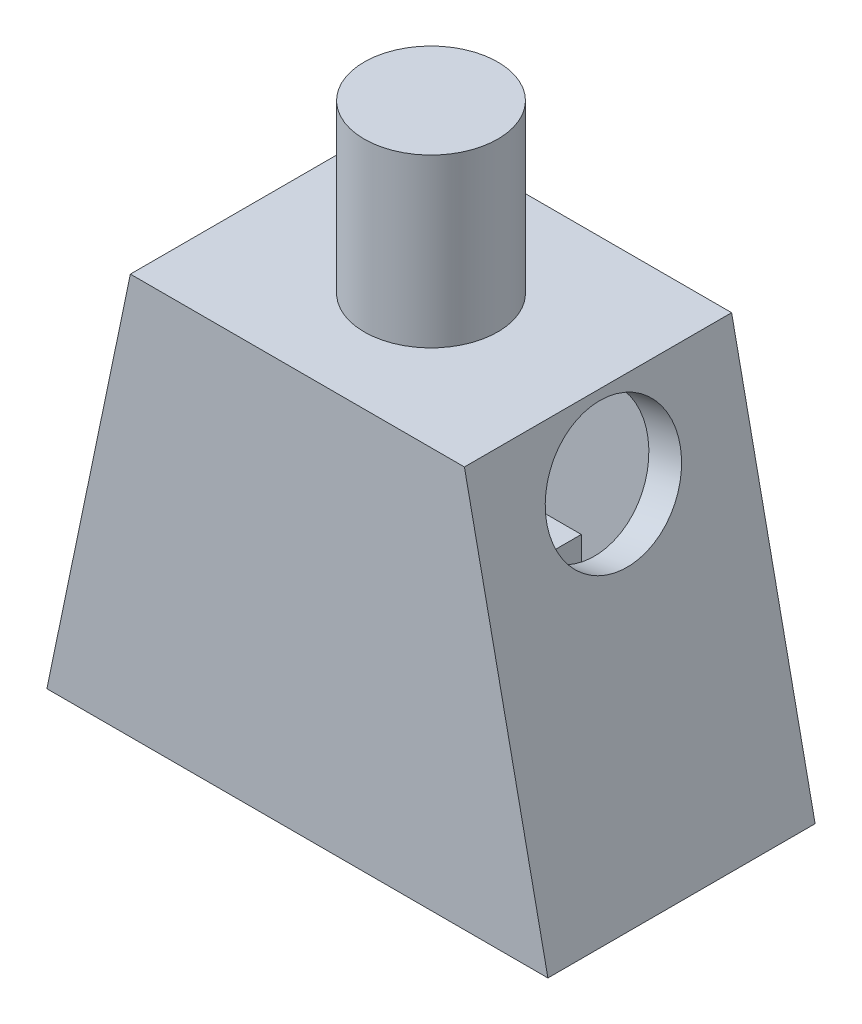
ISO-10303-21;
HEADER;
FILE_DESCRIPTION(('STEP AP214'),'2;1');
FILE_NAME('part.step','',(''),(''),'','','');
FILE_SCHEMA(('AUTOMOTIVE_DESIGN { 1 0 10303 214 1 1 1 1 }'));
ENDSEC;
DATA;
#1=APPLICATION_CONTEXT('core data for automotive mechanical design processes');
#2=APPLICATION_PROTOCOL_DEFINITION('international standard','automotive_design',2000,#1);
#3=PRODUCT_CONTEXT('',#1,'mechanical');
#4=PRODUCT('Part','Part','',(#3));
#5=PRODUCT_RELATED_PRODUCT_CATEGORY('part','',(#4));
#6=PRODUCT_DEFINITION_FORMATION('','',#4);
#7=PRODUCT_DEFINITION_CONTEXT('part definition',#1,'design');
#8=PRODUCT_DEFINITION('design','',#6,#7);
#9=PRODUCT_DEFINITION_SHAPE('','',#8);
#10=(LENGTH_UNIT() NAMED_UNIT(*) SI_UNIT(.MILLI.,.METRE.));
#11=(NAMED_UNIT(*) PLANE_ANGLE_UNIT() SI_UNIT($,.RADIAN.));
#12=(NAMED_UNIT(*) SI_UNIT($,.STERADIAN.) SOLID_ANGLE_UNIT());
#13=UNCERTAINTY_MEASURE_WITH_UNIT(LENGTH_MEASURE(1.E-05),#10,'distance_accuracy_value','');
#14=(GEOMETRIC_REPRESENTATION_CONTEXT(3) GLOBAL_UNCERTAINTY_ASSIGNED_CONTEXT((#13)) GLOBAL_UNIT_ASSIGNED_CONTEXT((#10,
#11,#12)) REPRESENTATION_CONTEXT('',''));
#15=CARTESIAN_POINT('',(0.,0.,0.));
#16=DIRECTION('',(0.,0.,1.));
#17=DIRECTION('',(1.,0.,0.));
#18=AXIS2_PLACEMENT_3D('',#15,#16,#17);
#19=CARTESIAN_POINT('',(0.,0.,-8.));
#20=DIRECTION('',(0.,-1.,0.));
#21=DIRECTION('',(0.,0.,-1.));
#22=AXIS2_PLACEMENT_3D('',#19,#20,#21);
#23=PLANE('',#22);
#24=DIRECTION('',(1.,0.,0.));
#25=VECTOR('',#24,1.);
#26=CARTESIAN_POINT('',(0.,0.,-7.));
#27=LINE('',#26,#25);
#28=CARTESIAN_POINT('',(9.,0.,-7.));
#29=VERTEX_POINT('',#28);
#30=CARTESIAN_POINT('',(13.9785291106557,0.,-7.));
#31=VERTEX_POINT('',#30);
#32=EDGE_CURVE('E199',#29,#31,#27,.T.);
#33=ORIENTED_EDGE('',*,*,#32,.F.);
#34=DIRECTION('',(0.,0.,1.));
#35=VECTOR('',#34,1.);
#36=CARTESIAN_POINT('',(9.,0.,-1.));
#37=LINE('',#36,#35);
#38=CARTESIAN_POINT('',(9.,0.,-1.));
#39=VERTEX_POINT('',#38);
#40=EDGE_CURVE('E292',#29,#39,#37,.T.);
#41=ORIENTED_EDGE('',*,*,#40,.T.);
#42=DIRECTION('',(1.,0.,0.));
#43=VECTOR('',#42,1.);
#44=CARTESIAN_POINT('',(0.,0.,-1.));
#45=LINE('',#44,#43);
#46=CARTESIAN_POINT('',(13.9785291106557,0.,-1.));
#47=VERTEX_POINT('',#46);
#48=EDGE_CURVE('E162',#39,#47,#45,.T.);
#49=ORIENTED_EDGE('',*,*,#48,.T.);
#50=DIRECTION('',(0.,0.,1.));
#51=VECTOR('',#50,1.);
#52=CARTESIAN_POINT('',(13.9785291106557,0.,-8.));
#53=LINE('',#52,#51);
#54=EDGE_CURVE('E220',#31,#47,#53,.T.);
#55=ORIENTED_EDGE('',*,*,#54,.F.);
#56=EDGE_LOOP('',(#33,#41,#49,#55));
#57=FACE_BOUND('',#56,.T.);
#58=DIRECTION('',(1.,0.,0.));
#59=VECTOR('',#58,1.);
#60=CARTESIAN_POINT('',(0.,0.,0.));
#61=LINE('',#60,#59);
#62=CARTESIAN_POINT('',(0.,0.,0.));
#63=VERTEX_POINT('',#62);
#64=CARTESIAN_POINT('',(15.,0.,0.));
#65=VERTEX_POINT('',#64);
#66=EDGE_CURVE('E239',#63,#65,#61,.T.);
#67=ORIENTED_EDGE('',*,*,#66,.F.);
#68=DIRECTION('',(0.,0.,1.));
#69=VECTOR('',#68,1.);
#70=CARTESIAN_POINT('',(0.,0.,-8.));
#71=LINE('',#70,#69);
#72=CARTESIAN_POINT('',(0.,0.,-8.));
#73=VERTEX_POINT('',#72);
#74=EDGE_CURVE('E43',#73,#63,#71,.T.);
#75=ORIENTED_EDGE('',*,*,#74,.F.);
#76=DIRECTION('',(1.,0.,0.));
#77=VECTOR('',#76,1.);
#78=CARTESIAN_POINT('',(0.,0.,-8.));
#79=LINE('',#78,#77);
#80=CARTESIAN_POINT('',(15.,0.,-8.));
#81=VERTEX_POINT('',#80);
#82=EDGE_CURVE('E226',#73,#81,#79,.T.);
#83=ORIENTED_EDGE('',*,*,#82,.T.);
#84=DIRECTION('',(0.,0.,1.));
#85=VECTOR('',#84,1.);
#86=CARTESIAN_POINT('',(15.,0.,-8.));
#87=LINE('',#86,#85);
#88=EDGE_CURVE('E249',#81,#65,#87,.T.);
#89=ORIENTED_EDGE('',*,*,#88,.T.);
#90=EDGE_LOOP('',(#67,#75,#83,#89));
#91=FACE_BOUND('',#90,.T.);
#92=DIRECTION('',(0.,0.,1.));
#93=VECTOR('',#92,1.);
#94=CARTESIAN_POINT('',(1.02147088934427,0.,-8.));
#95=LINE('',#94,#93);
#96=CARTESIAN_POINT('',(1.02147088934427,0.,-7.));
#97=VERTEX_POINT('',#96);
#98=CARTESIAN_POINT('',(1.02147088934427,0.,-1.));
#99=VERTEX_POINT('',#98);
#100=EDGE_CURVE('E209',#97,#99,#95,.T.);
#101=ORIENTED_EDGE('',*,*,#100,.T.);
#102=CARTESIAN_POINT('',(6.,0.,-1.));
#103=VERTEX_POINT('',#102);
#104=EDGE_CURVE('E212',#99,#103,#45,.T.);
#105=ORIENTED_EDGE('',*,*,#104,.T.);
#106=DIRECTION('',(0.,0.,-1.));
#107=VECTOR('',#106,1.);
#108=CARTESIAN_POINT('',(6.,0.,-1.));
#109=LINE('',#108,#107);
#110=CARTESIAN_POINT('',(6.,0.,-7.));
#111=VERTEX_POINT('',#110);
#112=EDGE_CURVE('E294',#103,#111,#109,.T.);
#113=ORIENTED_EDGE('',*,*,#112,.T.);
#114=EDGE_CURVE('E218',#97,#111,#27,.T.);
#115=ORIENTED_EDGE('',*,*,#114,.F.);
#116=EDGE_LOOP('',(#101,#105,#113,#115));
#117=FACE_BOUND('',#116,.T.);
#118=ADVANCED_FACE('F39',(#57,#91,#117),#23,.T.);
#119=CARTESIAN_POINT('',(2.5,12.,-8.));
#120=DIRECTION('',(-0.978980419737605,0.203954254112001,0.));
#121=DIRECTION('',(-0.203954254112001,-0.978980419737605,0.));
#122=AXIS2_PLACEMENT_3D('',#119,#120,#121);
#123=PLANE('',#122);
#124=CARTESIAN_POINT('',(2.03954254112001,9.78980419737605,-4.));
#125=DIRECTION('',(-0.978980419737605,0.203954254112001,0.));
#126=DIRECTION('',(-0.203954254112001,-0.978980419737605,0.));
#127=AXIS2_PLACEMENT_3D('',#124,#125,#126);
#128=CIRCLE('',#127,2.);
#129=CARTESIAN_POINT('',(1.63163403289601,7.83184335790084,-4.));
#130=VERTEX_POINT('',#129);
#131=EDGE_CURVE('E175',#130,#130,#128,.T.);
#132=ORIENTED_EDGE('',*,*,#131,.F.);
#133=EDGE_LOOP('',(#132));
#134=FACE_BOUND('',#133,.T.);
#135=DIRECTION('',(-0.203954254112001,-0.978980419737605,0.));
#136=VECTOR('',#135,1.);
#137=CARTESIAN_POINT('',(2.5,12.,0.));
#138=LINE('',#137,#136);
#139=CARTESIAN_POINT('',(2.5,12.,0.));
#140=VERTEX_POINT('',#139);
#141=EDGE_CURVE('E194',#140,#63,#138,.T.);
#142=ORIENTED_EDGE('',*,*,#141,.F.);
#143=DIRECTION('',(0.,0.,1.));
#144=VECTOR('',#143,1.);
#145=CARTESIAN_POINT('',(2.5,12.,-8.));
#146=LINE('',#145,#144);
#147=CARTESIAN_POINT('',(2.5,12.,-8.));
#148=VERTEX_POINT('',#147);
#149=EDGE_CURVE('E48',#148,#140,#146,.T.);
#150=ORIENTED_EDGE('',*,*,#149,.F.);
#151=DIRECTION('',(-0.203954254112001,-0.978980419737605,0.));
#152=VECTOR('',#151,1.);
#153=CARTESIAN_POINT('',(2.5,12.,-8.));
#154=LINE('',#153,#152);
#155=EDGE_CURVE('E222',#148,#73,#154,.T.);
#156=ORIENTED_EDGE('',*,*,#155,.T.);
#157=ORIENTED_EDGE('',*,*,#74,.T.);
#158=EDGE_LOOP('',(#142,#150,#156,#157));
#159=FACE_BOUND('',#158,.T.);
#160=ADVANCED_FACE('F41',(#134,#159),#123,.T.);
#161=CARTESIAN_POINT('',(12.5,12.,-8.));
#162=DIRECTION('',(0.,1.,0.));
#163=DIRECTION('',(0.,0.,1.));
#164=AXIS2_PLACEMENT_3D('',#161,#162,#163);
#165=PLANE('',#164);
#166=CARTESIAN_POINT('',(7.5,12.,-4.));
#167=DIRECTION('',(0.,1.,0.));
#168=DIRECTION('',(0.,0.,1.));
#169=AXIS2_PLACEMENT_3D('',#166,#167,#168);
#170=CIRCLE('',#169,2.);
#171=CARTESIAN_POINT('',(7.5,12.,-2.));
#172=VERTEX_POINT('',#171);
#173=EDGE_CURVE('E11',#172,#172,#170,.T.);
#174=ORIENTED_EDGE('',*,*,#173,.F.);
#175=EDGE_LOOP('',(#174));
#176=FACE_BOUND('',#175,.T.);
#177=DIRECTION('',(-1.,0.,0.));
#178=VECTOR('',#177,1.);
#179=CARTESIAN_POINT('',(12.5,12.,0.));
#180=LINE('',#179,#178);
#181=CARTESIAN_POINT('',(12.5,12.,0.));
#182=VERTEX_POINT('',#181);
#183=EDGE_CURVE('E230',#182,#140,#180,.T.);
#184=ORIENTED_EDGE('',*,*,#183,.F.);
#185=DIRECTION('',(0.,0.,1.));
#186=VECTOR('',#185,1.);
#187=CARTESIAN_POINT('',(12.5,12.,-8.));
#188=LINE('',#187,#186);
#189=CARTESIAN_POINT('',(12.5,12.,-8.));
#190=VERTEX_POINT('',#189);
#191=EDGE_CURVE('E248',#190,#182,#188,.T.);
#192=ORIENTED_EDGE('',*,*,#191,.F.);
#193=DIRECTION('',(-1.,0.,0.));
#194=VECTOR('',#193,1.);
#195=CARTESIAN_POINT('',(12.5,12.,-8.));
#196=LINE('',#195,#194);
#197=EDGE_CURVE('E232',#190,#148,#196,.T.);
#198=ORIENTED_EDGE('',*,*,#197,.T.);
#199=ORIENTED_EDGE('',*,*,#149,.T.);
#200=EDGE_LOOP('',(#184,#192,#198,#199));
#201=FACE_BOUND('',#200,.T.);
#202=ADVANCED_FACE('F262',(#176,#201),#165,.T.);
#203=CARTESIAN_POINT('',(15.,0.,-8.));
#204=DIRECTION('',(0.978980419737605,0.203954254112001,0.));
#205=DIRECTION('',(-0.203954254112001,0.978980419737605,0.));
#206=AXIS2_PLACEMENT_3D('',#203,#204,#205);
#207=PLANE('',#206);
#208=CARTESIAN_POINT('',(12.96045745888,9.78980419737605,-4.));
#209=DIRECTION('',(0.978980419737605,0.203954254112001,0.));
#210=DIRECTION('',(-0.203954254112001,0.978980419737605,0.));
#211=AXIS2_PLACEMENT_3D('',#208,#209,#210);
#212=CIRCLE('',#211,2.);
#213=CARTESIAN_POINT('',(12.552548950656,11.7477650368513,-4.));
#214=VERTEX_POINT('',#213);
#215=EDGE_CURVE('E177',#214,#214,#212,.T.);
#216=ORIENTED_EDGE('',*,*,#215,.F.);
#217=EDGE_LOOP('',(#216));
#218=FACE_BOUND('',#217,.T.);
#219=DIRECTION('',(-0.203954254112001,0.978980419737605,0.));
#220=VECTOR('',#219,1.);
#221=CARTESIAN_POINT('',(15.,0.,0.));
#222=LINE('',#221,#220);
#223=EDGE_CURVE('E243',#65,#182,#222,.T.);
#224=ORIENTED_EDGE('',*,*,#223,.F.);
#225=ORIENTED_EDGE('',*,*,#88,.F.);
#226=DIRECTION('',(-0.203954254112001,0.978980419737605,0.));
#227=VECTOR('',#226,1.);
#228=CARTESIAN_POINT('',(15.,0.,-8.));
#229=LINE('',#228,#227);
#230=EDGE_CURVE('E235',#81,#190,#229,.T.);
#231=ORIENTED_EDGE('',*,*,#230,.T.);
#232=ORIENTED_EDGE('',*,*,#191,.T.);
#233=EDGE_LOOP('',(#224,#225,#231,#232));
#234=FACE_BOUND('',#233,.T.);
#235=ADVANCED_FACE('F269',(#218,#234),#207,.T.);
#236=CARTESIAN_POINT('',(0.,0.,-8.));
#237=DIRECTION('',(0.,0.,1.));
#238=DIRECTION('',(1.,0.,0.));
#239=AXIS2_PLACEMENT_3D('',#236,#237,#238);
#240=PLANE('',#239);
#241=ORIENTED_EDGE('',*,*,#155,.F.);
#242=ORIENTED_EDGE('',*,*,#197,.F.);
#243=ORIENTED_EDGE('',*,*,#230,.F.);
#244=ORIENTED_EDGE('',*,*,#82,.F.);
#245=EDGE_LOOP('',(#241,#242,#243,#244));
#246=FACE_BOUND('',#245,.T.);
#247=ADVANCED_FACE('F268',(#246),#240,.F.);
#248=CARTESIAN_POINT('',(0.,0.,0.));
#249=DIRECTION('',(0.,0.,1.));
#250=DIRECTION('',(1.,0.,0.));
#251=AXIS2_PLACEMENT_3D('',#248,#249,#250);
#252=PLANE('',#251);
#253=ORIENTED_EDGE('',*,*,#141,.T.);
#254=ORIENTED_EDGE('',*,*,#66,.T.);
#255=ORIENTED_EDGE('',*,*,#223,.T.);
#256=ORIENTED_EDGE('',*,*,#183,.T.);
#257=EDGE_LOOP('',(#253,#254,#255,#256));
#258=FACE_BOUND('',#257,.T.);
#259=ADVANCED_FACE('F256',(#258),#252,.T.);
#260=CARTESIAN_POINT('',(3.47898041973761,11.796045745888,-8.));
#261=DIRECTION('',(-0.978980419737605,0.203954254112001,0.));
#262=DIRECTION('',(-0.203954254112001,-0.978980419737605,0.));
#263=AXIS2_PLACEMENT_3D('',#260,#261,#262);
#264=PLANE('',#263);
#265=DIRECTION('',(0.,0.,1.));
#266=VECTOR('',#265,1.);
#267=CARTESIAN_POINT('',(3.31313755601094,11.,-8.));
#268=LINE('',#267,#266);
#269=CARTESIAN_POINT('',(3.31313755601094,11.,-7.));
#270=VERTEX_POINT('',#269);
#271=CARTESIAN_POINT('',(3.31313755601094,11.,-5.38325046804848));
#272=VERTEX_POINT('',#271);
#273=EDGE_CURVE('E186',#270,#272,#268,.T.);
#274=ORIENTED_EDGE('',*,*,#273,.T.);
#275=CARTESIAN_POINT('',(3.01852296085761,9.58584994326405,-4.));
#276=DIRECTION('',(-0.978980419737605,0.203954254112001,0.));
#277=DIRECTION('',(-0.203954254112001,-0.978980419737605,0.));
#278=AXIS2_PLACEMENT_3D('',#275,#276,#277);
#279=CIRCLE('',#278,2.);
#280=CARTESIAN_POINT('',(3.31313755601094,11.,-2.61674953195152));
#281=VERTEX_POINT('',#280);
#282=EDGE_CURVE('E169',#281,#272,#279,.F.);
#283=ORIENTED_EDGE('',*,*,#282,.F.);
#284=CARTESIAN_POINT('',(3.31313755601094,11.,-1.));
#285=VERTEX_POINT('',#284);
#286=EDGE_CURVE('E192',#281,#285,#268,.T.);
#287=ORIENTED_EDGE('',*,*,#286,.T.);
#288=DIRECTION('',(-0.203954254112001,-0.978980419737605,0.));
#289=VECTOR('',#288,1.);
#290=CARTESIAN_POINT('',(0.978980419737604,-0.203954254112001,-1.));
#291=LINE('',#290,#289);
#292=EDGE_CURVE('E184',#285,#99,#291,.T.);
#293=ORIENTED_EDGE('',*,*,#292,.T.);
#294=ORIENTED_EDGE('',*,*,#100,.F.);
#295=DIRECTION('',(-0.203954254112001,-0.978980419737605,0.));
#296=VECTOR('',#295,1.);
#297=CARTESIAN_POINT('',(0.978980419737604,-0.203954254112001,-7.));
#298=LINE('',#297,#296);
#299=EDGE_CURVE('E195',#270,#97,#298,.T.);
#300=ORIENTED_EDGE('',*,*,#299,.F.);
#301=EDGE_LOOP('',(#274,#283,#287,#293,#294,#300));
#302=FACE_BOUND('',#301,.T.);
#303=ADVANCED_FACE('F306',(#302),#264,.F.);
#304=CARTESIAN_POINT('',(12.5,11.,-8.));
#305=DIRECTION('',(0.,1.,0.));
#306=DIRECTION('',(0.,0.,1.));
#307=AXIS2_PLACEMENT_3D('',#304,#305,#306);
#308=PLANE('',#307);
#309=ORIENTED_EDGE('',*,*,#286,.F.);
#310=CARTESIAN_POINT('',(-3.76939731147494,11.,-4.));
#311=DIRECTION('',(0.,1.,0.));
#312=DIRECTION('',(-1.,0.,0.));
#313=AXIS2_PLACEMENT_3D('',#310,#311,#312);
#314=ELLIPSE('',#313,9.80612053770501,2.);
#315=EDGE_CURVE('E171',#272,#281,#314,.F.);
#316=ORIENTED_EDGE('',*,*,#315,.F.);
#317=ORIENTED_EDGE('',*,*,#273,.F.);
#318=DIRECTION('',(-1.,0.,0.));
#319=VECTOR('',#318,1.);
#320=CARTESIAN_POINT('',(0.,11.,-7.));
#321=LINE('',#320,#319);
#322=CARTESIAN_POINT('',(11.6868624439891,11.,-7.));
#323=VERTEX_POINT('',#322);
#324=EDGE_CURVE('E207',#323,#270,#321,.T.);
#325=ORIENTED_EDGE('',*,*,#324,.F.);
#326=DIRECTION('',(0.,0.,1.));
#327=VECTOR('',#326,1.);
#328=CARTESIAN_POINT('',(11.6868624439891,11.,-8.));
#329=LINE('',#328,#327);
#330=CARTESIAN_POINT('',(11.6868624439891,11.,-5.38325046804849));
#331=VERTEX_POINT('',#330);
#332=EDGE_CURVE('E205',#323,#331,#329,.T.);
#333=ORIENTED_EDGE('',*,*,#332,.T.);
#334=CARTESIAN_POINT('',(18.7693973114749,11.,-4.));
#335=DIRECTION('',(0.,1.,0.));
#336=DIRECTION('',(1.,0.,0.));
#337=AXIS2_PLACEMENT_3D('',#334,#335,#336);
#338=ELLIPSE('',#337,9.80612053770501,2.);
#339=CARTESIAN_POINT('',(11.6868624439891,11.,-2.61674953195151));
#340=VERTEX_POINT('',#339);
#341=EDGE_CURVE('E180',#340,#331,#338,.F.);
#342=ORIENTED_EDGE('',*,*,#341,.F.);
#343=CARTESIAN_POINT('',(11.6868624439891,11.,-1.));
#344=VERTEX_POINT('',#343);
#345=EDGE_CURVE('E202',#340,#344,#329,.T.);
#346=ORIENTED_EDGE('',*,*,#345,.T.);
#347=DIRECTION('',(-1.,0.,0.));
#348=VECTOR('',#347,1.);
#349=CARTESIAN_POINT('',(0.,11.,-1.));
#350=LINE('',#349,#348);
#351=EDGE_CURVE('E197',#344,#285,#350,.T.);
#352=ORIENTED_EDGE('',*,*,#351,.T.);
#353=EDGE_LOOP('',(#309,#316,#317,#325,#333,#342,#346,#352));
#354=FACE_BOUND('',#353,.T.);
#355=ADVANCED_FACE('F315',(#354),#308,.F.);
#356=CARTESIAN_POINT('',(14.0210195802624,-0.203954254112001,-8.));
#357=DIRECTION('',(0.978980419737605,0.203954254112001,0.));
#358=DIRECTION('',(-0.203954254112001,0.978980419737605,0.));
#359=AXIS2_PLACEMENT_3D('',#356,#357,#358);
#360=PLANE('',#359);
#361=ORIENTED_EDGE('',*,*,#345,.F.);
#362=CARTESIAN_POINT('',(11.9814770391424,9.58584994326405,-4.));
#363=DIRECTION('',(0.978980419737605,0.203954254112001,0.));
#364=DIRECTION('',(-0.203954254112001,0.978980419737605,0.));
#365=AXIS2_PLACEMENT_3D('',#362,#363,#364);
#366=CIRCLE('',#365,2.);
#367=EDGE_CURVE('E172',#331,#340,#366,.F.);
#368=ORIENTED_EDGE('',*,*,#367,.F.);
#369=ORIENTED_EDGE('',*,*,#332,.F.);
#370=DIRECTION('',(-0.203954254112001,0.978980419737605,0.));
#371=VECTOR('',#370,1.);
#372=CARTESIAN_POINT('',(13.3970595137067,2.79105406535555,-7.));
#373=LINE('',#372,#371);
#374=EDGE_CURVE('E208',#31,#323,#373,.T.);
#375=ORIENTED_EDGE('',*,*,#374,.F.);
#376=ORIENTED_EDGE('',*,*,#54,.T.);
#377=DIRECTION('',(-0.203954254112001,0.978980419737605,0.));
#378=VECTOR('',#377,1.);
#379=CARTESIAN_POINT('',(13.3970595137067,2.79105406535555,-1.));
#380=LINE('',#379,#378);
#381=EDGE_CURVE('E203',#47,#344,#380,.T.);
#382=ORIENTED_EDGE('',*,*,#381,.T.);
#383=EDGE_LOOP('',(#361,#368,#369,#375,#376,#382));
#384=FACE_BOUND('',#383,.T.);
#385=ADVANCED_FACE('F317',(#384),#360,.F.);
#386=CARTESIAN_POINT('',(0.,0.,-7.));
#387=DIRECTION('',(0.,0.,1.));
#388=DIRECTION('',(1.,0.,0.));
#389=AXIS2_PLACEMENT_3D('',#386,#387,#388);
#390=PLANE('',#389);
#391=DIRECTION('',(0.,-1.,0.));
#392=VECTOR('',#391,1.);
#393=CARTESIAN_POINT('',(6.,5.,-7.));
#394=LINE('',#393,#392);
#395=CARTESIAN_POINT('',(6.,5.,-7.));
#396=VERTEX_POINT('',#395);
#397=EDGE_CURVE('E57',#396,#111,#394,.T.);
#398=ORIENTED_EDGE('',*,*,#397,.F.);
#399=DIRECTION('',(1.,0.,0.));
#400=VECTOR('',#399,1.);
#401=CARTESIAN_POINT('',(6.,5.,-7.));
#402=LINE('',#401,#400);
#403=CARTESIAN_POINT('',(9.,5.,-7.));
#404=VERTEX_POINT('',#403);
#405=EDGE_CURVE('E58',#396,#404,#402,.T.);
#406=ORIENTED_EDGE('',*,*,#405,.T.);
#407=DIRECTION('',(0.,-1.,0.));
#408=VECTOR('',#407,1.);
#409=CARTESIAN_POINT('',(9.,5.,-7.));
#410=LINE('',#409,#408);
#411=EDGE_CURVE('E156',#404,#29,#410,.T.);
#412=ORIENTED_EDGE('',*,*,#411,.T.);
#413=ORIENTED_EDGE('',*,*,#32,.T.);
#414=ORIENTED_EDGE('',*,*,#374,.T.);
#415=ORIENTED_EDGE('',*,*,#324,.T.);
#416=ORIENTED_EDGE('',*,*,#299,.T.);
#417=ORIENTED_EDGE('',*,*,#114,.T.);
#418=EDGE_LOOP('',(#398,#406,#412,#413,#414,#415,#416,#417));
#419=FACE_BOUND('',#418,.T.);
#420=ADVANCED_FACE('F295',(#419),#390,.T.);
#421=CARTESIAN_POINT('',(0.,0.,-1.));
#422=DIRECTION('',(0.,0.,1.));
#423=DIRECTION('',(1.,0.,0.));
#424=AXIS2_PLACEMENT_3D('',#421,#422,#423);
#425=PLANE('',#424);
#426=DIRECTION('',(-1.,0.,0.));
#427=VECTOR('',#426,1.);
#428=CARTESIAN_POINT('',(6.,5.,-1.));
#429=LINE('',#428,#427);
#430=CARTESIAN_POINT('',(9.,5.,-1.));
#431=VERTEX_POINT('',#430);
#432=CARTESIAN_POINT('',(6.,5.,-1.));
#433=VERTEX_POINT('',#432);
#434=EDGE_CURVE('E145',#431,#433,#429,.T.);
#435=ORIENTED_EDGE('',*,*,#434,.T.);
#436=DIRECTION('',(0.,-1.,0.));
#437=VECTOR('',#436,1.);
#438=CARTESIAN_POINT('',(6.,5.,-1.));
#439=LINE('',#438,#437);
#440=EDGE_CURVE('E161',#433,#103,#439,.T.);
#441=ORIENTED_EDGE('',*,*,#440,.T.);
#442=ORIENTED_EDGE('',*,*,#104,.F.);
#443=ORIENTED_EDGE('',*,*,#292,.F.);
#444=ORIENTED_EDGE('',*,*,#351,.F.);
#445=ORIENTED_EDGE('',*,*,#381,.F.);
#446=ORIENTED_EDGE('',*,*,#48,.F.);
#447=DIRECTION('',(0.,-1.,0.));
#448=VECTOR('',#447,1.);
#449=CARTESIAN_POINT('',(9.,5.,-1.));
#450=LINE('',#449,#448);
#451=EDGE_CURVE('E158',#431,#39,#450,.T.);
#452=ORIENTED_EDGE('',*,*,#451,.F.);
#453=EDGE_LOOP('',(#435,#441,#442,#443,#444,#445,#446,#452));
#454=FACE_BOUND('',#453,.T.);
#455=ADVANCED_FACE('F157',(#454),#425,.F.);
#456=CARTESIAN_POINT('',(7.5,17.,-4.));
#457=DIRECTION('',(0.,-1.,0.));
#458=DIRECTION('',(0.,0.,-1.));
#459=AXIS2_PLACEMENT_3D('',#456,#457,#458);
#460=CYLINDRICAL_SURFACE('',#459,2.);
#461=CARTESIAN_POINT('',(7.5,17.,-4.));
#462=DIRECTION('',(0.,1.,0.));
#463=DIRECTION('',(0.,0.,1.));
#464=AXIS2_PLACEMENT_3D('',#461,#462,#463);
#465=CIRCLE('',#464,2.);
#466=CARTESIAN_POINT('',(7.5,17.,-2.));
#467=VERTEX_POINT('',#466);
#468=EDGE_CURVE('E182',#467,#467,#465,.T.);
#469=ORIENTED_EDGE('',*,*,#468,.F.);
#470=EDGE_LOOP('',(#469));
#471=FACE_BOUND('',#470,.T.);
#472=ORIENTED_EDGE('',*,*,#173,.T.);
#473=EDGE_LOOP('',(#472));
#474=FACE_BOUND('',#473,.T.);
#475=ADVANCED_FACE('F326',(#471,#474),#460,.T.);
#476=CARTESIAN_POINT('',(7.5,17.,-4.));
#477=DIRECTION('',(0.,1.,0.));
#478=DIRECTION('',(0.,0.,1.));
#479=AXIS2_PLACEMENT_3D('',#476,#477,#478);
#480=PLANE('',#479);
#481=ORIENTED_EDGE('',*,*,#468,.T.);
#482=EDGE_LOOP('',(#481));
#483=FACE_BOUND('',#482,.T.);
#484=ADVANCED_FACE('F322',(#483),#480,.T.);
#485=CARTESIAN_POINT('',(-1.4167405444478,6.79455461334943,-4.));
#486=DIRECTION('',(0.978980419737605,0.203954254112001,0.));
#487=DIRECTION('',(-0.203954254112001,0.978980419737605,0.));
#488=AXIS2_PLACEMENT_3D('',#485,#486,#487);
#489=CYLINDRICAL_SURFACE('',#488,2.);
#490=ORIENTED_EDGE('',*,*,#215,.T.);
#491=EDGE_LOOP('',(#490));
#492=FACE_BOUND('',#491,.T.);
#493=ORIENTED_EDGE('',*,*,#341,.T.);
#494=ORIENTED_EDGE('',*,*,#367,.T.);
#495=EDGE_LOOP('',(#493,#494));
#496=FACE_BOUND('',#495,.T.);
#497=ADVANCED_FACE('F318',(#492,#496),#489,.F.);
#498=CARTESIAN_POINT('',(16.4167405444478,6.79455461334943,-4.));
#499=DIRECTION('',(-0.978980419737605,0.203954254112001,0.));
#500=DIRECTION('',(-0.203954254112001,-0.978980419737605,0.));
#501=AXIS2_PLACEMENT_3D('',#498,#499,#500);
#502=CYLINDRICAL_SURFACE('',#501,2.);
#503=ORIENTED_EDGE('',*,*,#131,.T.);
#504=EDGE_LOOP('',(#503));
#505=FACE_BOUND('',#504,.T.);
#506=ORIENTED_EDGE('',*,*,#282,.T.);
#507=ORIENTED_EDGE('',*,*,#315,.T.);
#508=EDGE_LOOP('',(#506,#507));
#509=FACE_BOUND('',#508,.T.);
#510=ADVANCED_FACE('F324',(#505,#509),#502,.F.);
#511=CARTESIAN_POINT('',(6.,5.,-1.));
#512=DIRECTION('',(-1.,0.,0.));
#513=DIRECTION('',(0.,0.,1.));
#514=AXIS2_PLACEMENT_3D('',#511,#512,#513);
#515=PLANE('',#514);
#516=ORIENTED_EDGE('',*,*,#112,.F.);
#517=ORIENTED_EDGE('',*,*,#440,.F.);
#518=DIRECTION('',(0.,0.,-1.));
#519=VECTOR('',#518,1.);
#520=CARTESIAN_POINT('',(6.,5.,-1.));
#521=LINE('',#520,#519);
#522=EDGE_CURVE('E149',#433,#396,#521,.T.);
#523=ORIENTED_EDGE('',*,*,#522,.T.);
#524=ORIENTED_EDGE('',*,*,#397,.T.);
#525=EDGE_LOOP('',(#516,#517,#523,#524));
#526=FACE_BOUND('',#525,.T.);
#527=ADVANCED_FACE('F301',(#526),#515,.T.);
#528=CARTESIAN_POINT('',(9.,5.,-1.));
#529=DIRECTION('',(1.,0.,0.));
#530=DIRECTION('',(0.,0.,-1.));
#531=AXIS2_PLACEMENT_3D('',#528,#529,#530);
#532=PLANE('',#531);
#533=ORIENTED_EDGE('',*,*,#40,.F.);
#534=ORIENTED_EDGE('',*,*,#411,.F.);
#535=DIRECTION('',(0.,0.,1.));
#536=VECTOR('',#535,1.);
#537=CARTESIAN_POINT('',(9.,5.,-1.));
#538=LINE('',#537,#536);
#539=EDGE_CURVE('E143',#404,#431,#538,.T.);
#540=ORIENTED_EDGE('',*,*,#539,.T.);
#541=ORIENTED_EDGE('',*,*,#451,.T.);
#542=EDGE_LOOP('',(#533,#534,#540,#541));
#543=FACE_BOUND('',#542,.T.);
#544=ADVANCED_FACE('F151',(#543),#532,.T.);
#545=CARTESIAN_POINT('',(0.,5.,0.));
#546=DIRECTION('',(0.,1.,0.));
#547=DIRECTION('',(0.,0.,1.));
#548=AXIS2_PLACEMENT_3D('',#545,#546,#547);
#549=PLANE('',#548);
#550=ORIENTED_EDGE('',*,*,#405,.F.);
#551=ORIENTED_EDGE('',*,*,#522,.F.);
#552=ORIENTED_EDGE('',*,*,#434,.F.);
#553=ORIENTED_EDGE('',*,*,#539,.F.);
#554=EDGE_LOOP('',(#550,#551,#552,#553));
#555=FACE_BOUND('',#554,.T.);
#556=ADVANCED_FACE('F144',(#555),#549,.T.);
#557=CLOSED_SHELL('',(#118,#160,#202,#235,#247,#259,#303,#355,#385,#420,#455,#475,#484,#497,
#510,#527,#544,#556));
#558=MANIFOLD_SOLID_BREP('B2',#557);
#559=ADVANCED_BREP_SHAPE_REPRESENTATION('',(#18,#558),#14);
#560=SHAPE_DEFINITION_REPRESENTATION(#9,#559);
ENDSEC;
END-ISO-10303-21;
